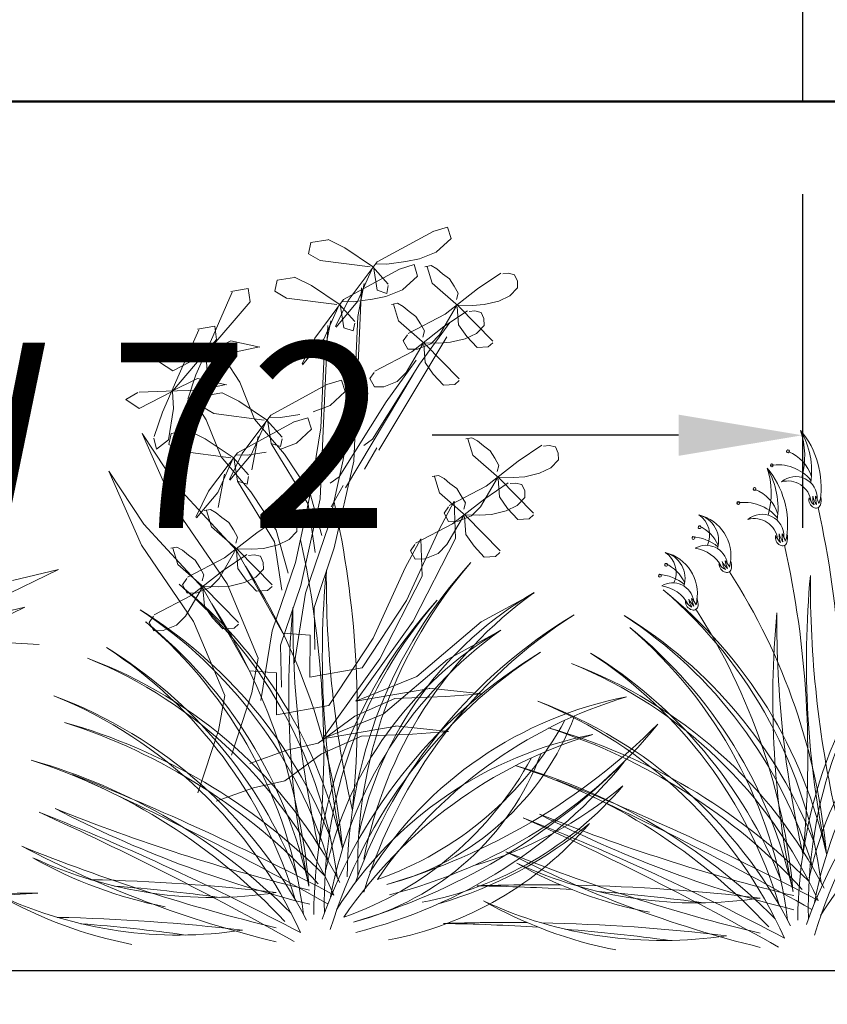
# Model space of a CAD drawing. Units: inches. Extents: x 89 to 490, y -59 to 378.
# Tile 11 of 20: x 374 to 400, y -24 to 7. Entities that reach past the tile are written whole.
import ezdxf

# ---------------------------------------------------------------- set-up
doc = ezdxf.new("R2010")
doc.units = ezdxf.units.IN
doc.header["$MEASUREMENT"] = 0
for name, color, linetype, lineweight in [('A-ANNO-DIMS', 2, 'Continuous', 18), ('L-PLNT', 94, 'Continuous', 18), ('L-PLNT-EDGE', 31, 'Continuous', 25), ('Outer Walls', 12, 'Continuous', 50), ('Windows', 171, 'Continuous', 25)]:
    doc.layers.add(name, color=color, linetype=linetype, lineweight=lineweight)
doc.layers.add('fl', color=73, linetype='Continuous', lineweight=9, true_color=0xa3d166)
doc.styles.get("Standard").update_dxf_attribs({"font": 'arial.ttf'})
doc.dimstyles.get("Standard").update_dxf_attribs({"dimtxt": 6, "dimasz": 4, "dimexe": 3, "dimexo": 3, "dimgap": 0.09, "dimtad": 0, "dimtih": 1, "dimtoh": 1, "dimdec": 1, "dimzin": 0, "dimdsep": 46, "dimlunit": 3, "dimtxsty": 'Standard', "dimcen": 0.09, "dimadec": 0, "dimazin": 0, "dimtfac": 1, "dimtdec": 1, "dimtofl": 0, "dimtmove": 0, "dimatfit": 3, "dimfxl": 1, "dimtolj": 1, "dimtzin": 0, "dimarcsym": 0})

# ---------------------------------------------------------------- blocks, each defined once
blk = doc.blocks.new('Window')
blk.add_lwpolyline([(588.369, 99.053), (588.369, 90.053), (516.369, 90.053), (516.369, 99.053)], close=True)
blk = doc.blocks.new('Plantation')
at = {"layer": 'fl'}
for p, q in [((609.786, 34.419), (611.6, 35.405)), ((612.07, 35.547), (611.594, 35.406)), ((612.182, 35.177), (612.07, 35.547)), ((608.2, 35.134), (607.643, 35.044)), ((608.206, 35.143), (608.75, 34.87)), ((611.699, 34.73), (612.182, 35.177)), ((607.643, 35.044), (607.57, 34.684)), ((608.75, 34.87), (609.645, 34.268)), ((611.158, 34.521), (611.699, 34.73)), ((607.57, 34.684), (607.946, 34.465)), ((607.946, 34.465), (609.569, 34.254)), ((608.856, 33.172), (609.786, 34.419)), ((610.099, 34.343), (610.721, 34.434)), ((610.721, 34.434), (611.158, 34.521)), ((608.702, 33.201), (610.516, 34.186)), ((609.151, 33.131), (609.649, 34.242)), ((609.645, 34.268), (610.151, 33.702)), ((609.795, 33.501), (609.675, 34.269)), ((609.754, 34.35), (610.099, 34.343)), ((610.986, 34.329), (610.51, 34.188)), ((611.099, 33.959), (610.986, 34.329)), ((611.337, 34.257), (611.537, 34.297)), ((611.405, 34.263), (611.569, 33.734)), ((611.537, 34.297), (611.721, 34.191)), ((611.721, 34.191), (611.905, 34.03)), ((606.56, 33.826), (606.486, 33.466)), ((607.116, 33.916), (606.56, 33.826)), ((607.122, 33.925), (607.666, 33.652)), ((610.615, 33.512), (611.099, 33.959)), ((611.905, 34.03), (612.126, 33.87)), ((612.126, 33.87), (612.276, 33.636)), ((613.034, 33.541), (613.794, 34.053)), ((614.034, 34.049), (613.852, 34.028)), ((614.235, 33.998), (614.034, 34.049)), ((614.329, 33.799), (614.235, 33.998)), ((614.333, 33.581), (614.329, 33.799)), ((605.062, 33.457), (605.625, 33.555)), ((605.625, 33.555), (605.683, 33.128)), ((606.486, 33.466), (606.862, 33.247)), ((607.666, 33.652), (608.561, 33.05)), ((609.28, 33.582), (609.036, 27.974)), ((609.166, 32.648), (609.372, 33.724)), ((610.102, 33.4), (609.795, 33.501)), ((610.074, 33.303), (610.615, 33.512)), ((610.151, 33.653), (610.102, 33.4)), ((611.569, 33.734), (612.421, 32.985)), ((611.992, 32.728), (613.034, 33.541)), ((612.276, 33.636), (612.408, 33.402)), ((614.083, 33.322), (614.333, 33.581)), ((604.472, 32.002), (605.104, 33.433)), ((606.862, 33.247), (608.486, 33.036)), ((607.772, 31.954), (608.702, 33.201)), ((608.447, 32.332), (608.856, 33.172)), ((609.015, 33.125), (609.638, 33.216)), ((609.638, 33.216), (610.074, 33.303)), ((612.408, 33.402), (612.356, 33.201)), ((613.251, 33.034), (613.722, 33.152)), ((613.722, 33.152), (614.083, 33.322)), ((605.683, 33.128), (604.255, 31.456)), ((608.067, 31.913), (608.565, 33.024)), ((608.461, 32.308), (609.151, 33.131)), ((608.561, 33.05), (609.067, 32.484)), ((608.711, 32.283), (608.591, 33.051)), ((608.67, 33.132), (609.015, 33.125)), ((610.254, 33.039), (610.453, 33.079)), ((610.321, 33.045), (610.485, 32.516)), ((610.453, 33.079), (610.637, 32.973)), ((610.637, 32.973), (610.821, 32.812)), ((611.812, 32.062), (612.36, 33)), ((611.95, 32.323), (612.71, 32.835)), ((612.379, 32.964), (612.425, 32.382)), ((612.414, 33.019), (612.869, 33.009)), ((612.421, 32.985), (613.528, 31.857)), ((612.95, 32.831), (612.768, 32.81)), ((612.869, 33.009), (613.251, 33.034)), ((613.151, 32.78), (612.95, 32.831)), ((608.082, 31.43), (608.288, 32.506)), ((609.053, 30.262), (609.166, 32.648)), ((610.485, 32.516), (611.337, 31.767)), ((610.798, 32.104), (611.992, 32.728)), ((610.821, 32.812), (611.043, 32.652)), ((611.043, 32.652), (611.192, 32.418)), ((613.245, 32.581), (613.151, 32.78)), ((613.249, 32.363), (613.245, 32.581)), ((603.389, 30.784), (604.02, 32.215)), ((603.978, 32.239), (604.541, 32.337)), ((604.541, 32.337), (604.599, 31.91)), ((608.196, 32.364), (607.953, 26.756)), ((609.018, 32.182), (608.711, 32.283)), ((609.067, 32.435), (609.018, 32.182)), ((610.908, 31.51), (611.95, 32.323)), ((611.163, 31.112), (612.138, 32.457)), ((611.192, 32.418), (611.324, 32.184)), ((611.324, 32.184), (611.273, 31.982)), ((612.425, 32.382), (612.687, 32.004)), ((612.999, 32.104), (613.249, 32.363)), ((604.599, 31.91), (603.171, 30.238)), ((603.931, 30.768), (604.472, 32.002)), ((607.364, 31.114), (607.772, 31.954)), ((607.378, 31.09), (608.067, 31.913)), ((609.85, 28.33), (612.039, 31.99)), ((610.775, 32.062), (610.633, 31.859)), ((611.526, 31.766), (611.812, 32.062)), ((612.167, 31.816), (612.638, 31.933)), ((612.638, 31.933), (612.999, 32.104)), ((612.687, 32.004), (613.02, 31.646)), ((605.064, 31.86), (604.217, 31.443)), ((605.998, 31.662), (605.064, 31.86)), ((605.122, 31.489), (605.991, 31.665)), ((610.633, 31.859), (610.784, 31.589)), ((610.728, 30.844), (611.276, 31.782)), ((610.784, 31.589), (611.093, 31.594)), ((611.093, 31.594), (611.526, 31.766)), ((611.295, 31.746), (611.341, 31.164)), ((611.33, 31.801), (611.785, 31.791)), ((611.337, 31.767), (612.445, 30.639)), ((611.785, 31.791), (612.167, 31.816)), ((613.02, 31.646), (613.384, 31.671)), ((613.384, 31.671), (613.527, 31.801)), ((603.137, 31.411), (602.752, 31.178)), ((603.18, 31.423), (604.054, 31.453)), ((603.184, 30.896), (604.242, 31.443)), ((604.054, 31.453), (605.122, 31.489)), ((604.29, 30.89), (604.255, 31.443)), ((604.887, 31.238), (605.349, 30.525)), ((607.969, 29.044), (608.082, 31.43)), ((609.714, 30.886), (610.908, 31.51)), ((610.079, 29.894), (611.054, 31.239)), ((602.752, 31.178), (603.184, 30.896)), ((609.641, 28.678), (611.163, 31.112)), ((611.341, 31.164), (611.603, 30.786)), ((602.847, 29.55), (603.389, 30.784)), ((603.98, 30.642), (603.133, 30.224)), ((603.666, 29.981), (603.931, 30.768)), ((604.914, 30.444), (603.98, 30.642)), ((604.131, 29.882), (604.29, 30.89)), ((608.638, 30.589), (608.162, 30.448)), ((608.751, 30.219), (608.638, 30.589)), ((608.766, 27.112), (610.956, 30.772)), ((609.692, 30.844), (609.55, 30.641)), ((609.55, 30.641), (609.7, 30.371)), ((610.443, 30.548), (610.728, 30.844)), ((611.603, 30.786), (611.936, 30.428)), ((602.97, 30.235), (604.038, 30.271)), ((604.038, 30.271), (604.907, 30.447)), ((605.349, 30.525), (605.828, 29.326)), ((606.354, 29.461), (608.168, 30.447)), ((609.7, 30.371), (610.009, 30.376)), ((610.009, 30.376), (610.443, 30.548)), ((611.936, 30.428), (612.3, 30.453)), ((612.3, 30.453), (612.443, 30.583)), ((602.053, 30.193), (601.668, 29.96)), ((601.668, 29.96), (602.1, 29.678)), ((602.096, 30.205), (602.97, 30.235)), ((602.1, 29.678), (603.158, 30.225)), ((603.206, 29.672), (603.171, 30.225)), ((603.804, 30.02), (604.265, 29.307)), ((604.212, 30.086), (604.138, 29.726)), ((604.768, 30.176), (604.212, 30.086)), ((604.774, 30.185), (605.318, 29.912)), ((608.267, 29.772), (608.751, 30.219)), ((608.692, 28.013), (609.053, 30.262)), ((603.047, 28.664), (603.206, 29.672)), ((603.653, 29.936), (603.735, 29.573)), ((603.735, 29.573), (604.131, 29.882)), ((604.138, 29.726), (604.514, 29.507)), ((605.318, 29.912), (606.213, 29.31)), ((607.726, 29.563), (608.267, 29.772)), ((608.558, 27.46), (610.079, 29.894)), ((602.582, 28.763), (602.847, 29.55)), ((604.514, 29.507), (606.138, 29.296)), ((605.424, 28.214), (606.354, 29.461)), ((605.828, 29.326), (606.79, 28.192)), ((606.322, 29.392), (606.667, 29.385)), ((606.667, 29.385), (607.29, 29.476)), ((607.554, 29.371), (607.079, 29.23)), ((607.667, 29.001), (607.554, 29.371)), ((604.265, 29.307), (604.744, 28.108)), ((605.27, 28.243), (607.084, 29.229)), ((605.719, 28.173), (606.217, 29.284)), ((606.213, 29.31), (606.719, 28.744)), ((606.363, 28.543), (606.244, 29.311)), ((607.183, 28.554), (607.667, 29.001)), ((607.608, 26.795), (607.969, 29.044)), ((603.251, 26.467), (602.197, 28.861)), ((602.197, 28.861), (603.325, 27.15)), ((602.569, 28.718), (602.651, 28.355)), ((603.128, 28.868), (603.054, 28.508)), ((603.684, 28.958), (603.128, 28.868)), ((603.69, 28.967), (604.234, 28.694)), ((604.234, 28.694), (605.13, 28.092)), ((605.734, 27.69), (605.94, 28.766)), ((606.719, 28.695), (606.67, 28.442)), ((609.357, 28.474), (609.641, 28.678)), ((612.657, 28.689), (612.857, 28.729)), ((612.724, 28.695), (612.888, 28.166)), ((612.857, 28.729), (613.04, 28.623)), ((602.651, 28.355), (603.047, 28.664)), ((603.054, 28.508), (603.43, 28.289)), ((606.363, 28.543), (607.558, 26.582)), ((606.67, 28.442), (606.363, 28.543)), ((606.643, 28.345), (607.183, 28.554)), ((609.383, 27.707), (609.78, 28.397)), ((613.04, 28.623), (613.225, 28.462)), ((613.225, 28.462), (613.446, 28.302)), ((614.353, 27.973), (615.114, 28.485)), ((615.353, 28.481), (615.172, 28.46)), ((615.554, 28.43), (615.353, 28.481)), ((615.649, 28.231), (615.554, 28.43)), ((603.43, 28.289), (605.054, 28.078)), ((604.341, 26.996), (605.27, 28.243)), ((604.635, 26.955), (605.134, 28.066)), ((604.744, 28.108), (605.706, 26.974)), ((605.016, 27.374), (605.424, 28.214)), ((605.03, 27.35), (605.719, 28.173)), ((605.13, 28.092), (605.635, 27.526)), ((605.279, 27.325), (605.16, 28.093)), ((605.238, 28.174), (605.583, 28.167)), ((605.583, 28.167), (606.206, 28.258)), ((606.79, 28.192), (607.61, 26.956)), ((612.888, 28.166), (613.74, 27.418)), ((613.446, 28.302), (613.596, 28.068)), ((613.596, 28.068), (613.727, 27.834)), ((615.653, 28.013), (615.649, 28.231)), ((608.229, 25.907), (608.692, 28.013)), ((609.036, 27.974), (608.403, 25.161)), ((613.312, 27.16), (614.353, 27.973)), ((613.727, 27.834), (613.676, 27.633)), ((615.042, 27.584), (615.402, 27.754)), ((615.402, 27.754), (615.653, 28.013)), ((602.168, 25.249), (601.114, 27.643)), ((601.114, 27.643), (602.241, 25.932)), ((604.65, 26.472), (604.857, 27.548)), ((605.635, 27.477), (605.587, 27.224)), ((608.273, 27.256), (608.558, 27.46)), ((611.573, 27.471), (611.773, 27.511)), ((611.641, 27.477), (611.804, 26.948)), ((611.773, 27.511), (611.957, 27.405)), ((611.957, 27.405), (612.141, 27.244)), ((613.132, 26.494), (613.68, 27.432)), ((613.734, 27.451), (614.189, 27.441)), ((613.74, 27.418), (614.848, 26.289)), ((614.189, 27.441), (614.571, 27.466)), ((614.571, 27.466), (615.042, 27.584)), ((603.325, 27.15), (605.243, 25.076)), ((605.279, 27.325), (606.475, 25.364)), ((605.587, 27.224), (605.279, 27.325)), ((608.299, 26.489), (608.696, 27.179)), ((612.118, 26.536), (613.312, 27.16)), ((612.141, 27.244), (612.362, 27.084)), ((612.362, 27.084), (612.512, 26.85)), ((613.269, 26.755), (614.03, 27.267)), ((613.699, 27.396), (613.745, 26.814)), ((614.269, 27.263), (614.088, 27.242)), ((614.47, 27.212), (614.269, 27.263)), ((614.565, 27.013), (614.47, 27.212)), ((603.932, 26.156), (604.341, 26.996)), ((603.946, 26.132), (604.635, 26.955)), ((605.706, 26.974), (606.526, 25.738)), ((607.145, 24.689), (607.608, 26.795)), ((607.61, 26.956), (607.998, 25.559)), ((611.804, 26.948), (612.656, 26.2)), ((612.512, 26.85), (612.643, 26.616)), ((613.745, 26.814), (614.006, 26.437)), ((614.319, 26.536), (614.569, 26.795)), ((614.569, 26.795), (614.565, 27.013)), ((604.94, 23.997), (603.251, 26.467)), ((607.953, 26.756), (607.319, 23.943)), ((607.558, 26.582), (607.791, 25.014)), ((611.783, 25.737), (612.286, 26.678)), ((612.095, 26.494), (611.953, 26.291)), ((612.228, 25.942), (613.269, 26.755)), ((612.286, 26.678), (612.328, 25.464)), ((612.643, 26.616), (612.592, 26.415)), ((612.846, 26.198), (613.132, 26.494)), ((613.958, 26.366), (614.319, 26.536)), ((604.202, 26.369), (604.401, 26.409)), ((604.269, 26.376), (604.433, 25.846)), ((604.401, 26.409), (604.585, 26.303)), ((604.585, 26.303), (604.77, 26.142)), ((604.77, 26.142), (604.991, 25.982)), ((605.898, 25.653), (606.658, 26.165)), ((606.898, 26.161), (606.717, 26.14)), ((607.099, 26.11), (606.898, 26.161)), ((611.953, 26.291), (612.103, 26.021)), ((612.048, 25.276), (612.596, 26.214)), ((612.413, 26.026), (612.846, 26.198)), ((612.615, 26.178), (612.661, 25.596)), ((612.65, 26.233), (613.105, 26.223)), ((612.656, 26.2), (613.764, 25.071)), ((613.105, 26.223), (613.487, 26.248)), ((613.487, 26.248), (613.958, 26.366)), ((614.006, 26.437), (614.34, 26.078)), ((614.704, 26.103), (614.847, 26.233)), ((602.241, 25.932), (604.159, 23.858)), ((604.433, 25.846), (605.285, 25.098)), ((604.991, 25.982), (605.141, 25.748)), ((607.194, 25.912), (607.099, 26.11)), ((607.197, 25.693), (607.194, 25.912)), ((607.478, 23.694), (608.229, 25.907)), ((611.034, 25.318), (612.228, 25.942)), ((612.103, 26.021), (612.413, 26.026)), ((614.34, 26.078), (614.704, 26.103)), ((604.856, 24.84), (605.898, 25.653)), ((605.141, 25.748), (605.272, 25.514)), ((605.272, 25.514), (605.221, 25.313)), ((606.526, 25.738), (606.914, 24.341)), ((606.947, 25.434), (607.197, 25.693)), ((610.743, 23.465), (611.783, 25.737)), ((612.661, 25.596), (612.923, 25.219)), ((603.856, 22.778), (602.168, 25.249)), ((603.118, 25.151), (603.318, 25.191)), ((603.318, 25.191), (603.501, 25.085)), ((606.115, 25.146), (606.586, 25.264)), ((606.475, 25.364), (606.707, 23.796)), ((606.586, 25.264), (606.947, 25.434)), ((610.7, 24.519), (611.202, 25.46)), ((611.011, 25.276), (610.869, 25.073)), ((612.328, 25.464), (610.96, 22.792)), ((611.202, 25.46), (611.244, 24.246)), ((611.762, 24.98), (612.048, 25.276)), ((612.923, 25.219), (613.256, 24.86)), ((603.185, 25.158), (603.349, 24.628)), ((603.501, 25.085), (603.686, 24.924)), ((603.686, 24.924), (603.907, 24.764)), ((604.677, 24.174), (605.224, 25.112)), ((604.814, 24.435), (605.575, 24.947)), ((605.243, 25.076), (606.744, 22.405)), ((605.243, 25.076), (605.29, 24.494)), ((605.279, 25.132), (605.734, 25.121)), ((605.285, 25.098), (606.393, 23.969)), ((605.814, 24.943), (605.633, 24.922)), ((605.734, 25.121), (606.115, 25.146)), ((606.015, 24.892), (605.814, 24.943)), ((606.11, 24.694), (606.015, 24.892)), ((608.403, 25.161), (607.753, 23.236)), ((610.869, 25.073), (611.02, 24.803)), ((611.329, 24.808), (611.762, 24.98)), ((613.256, 24.86), (613.62, 24.885)), ((613.62, 24.885), (613.763, 25.015)), ((603.349, 24.628), (604.201, 23.88)), ((603.662, 24.216), (604.856, 24.84)), ((603.907, 24.764), (604.057, 24.53)), ((606.113, 24.475), (606.11, 24.694)), ((606.394, 22.476), (607.145, 24.689)), ((611.02, 24.803), (611.329, 24.808)), ((599.485, 24.463), (597.342, 23.428)), ((597.995, 24.105), (599.485, 24.463)), ((603.772, 23.622), (604.814, 24.435)), ((604.057, 24.53), (604.188, 24.296)), ((604.188, 24.296), (604.137, 24.095)), ((605.29, 24.494), (605.551, 24.117)), ((605.502, 24.046), (605.863, 24.216)), ((605.863, 24.216), (606.113, 24.475)), ((609.659, 22.247), (610.7, 24.519)), ((611.244, 24.246), (609.876, 21.574)), ((603.64, 24.174), (603.498, 23.972)), ((603.498, 23.972), (603.648, 23.701)), ((604.195, 23.914), (604.65, 23.903)), ((604.391, 23.878), (604.677, 24.174)), ((604.65, 23.903), (605.031, 23.928)), ((605.945, 21.6), (604.94, 23.997)), ((605.031, 23.928), (605.502, 24.046)), ((605.551, 24.117), (605.885, 23.758)), ((606.248, 23.783), (606.392, 23.913)), ((607.319, 23.943), (606.669, 22.018)), ((602.578, 22.998), (603.772, 23.622)), ((603.593, 22.956), (604.141, 23.894)), ((603.648, 23.701), (603.957, 23.706)), ((603.957, 23.706), (604.391, 23.878)), ((604.159, 23.858), (605.66, 21.187)), ((604.159, 23.858), (604.206, 23.276)), ((604.201, 23.88), (605.309, 22.751)), ((605.885, 23.758), (606.248, 23.783)), ((607.117, 21.446), (607.478, 23.694)), ((613.149, 22.769), (614.867, 23.703)), ((604.206, 23.276), (604.467, 22.899)), ((609.31, 21.277), (610.743, 23.465)), ((598.401, 23.245), (596.258, 22.21)), ((596.911, 22.887), (598.401, 23.245)), ((602.556, 22.956), (602.414, 22.754)), ((603.307, 22.66), (603.593, 22.956)), ((607.753, 23.236), (607.777, 21.87)), ((602.414, 22.754), (602.564, 22.483)), ((602.874, 22.488), (603.307, 22.66)), ((604.861, 20.382), (603.856, 22.778)), ((604.467, 22.899), (604.801, 22.54)), ((605.164, 22.565), (605.308, 22.695)), ((610.96, 22.792), (609.104, 20.201)), ((611.07, 20.997), (613.149, 22.769)), ((602.564, 22.483), (602.874, 22.488)), ((604.801, 22.54), (605.164, 22.565)), ((606.033, 20.228), (606.394, 22.476)), ((606.744, 22.405), (607.621, 22.338)), ((607.621, 22.338), (607.619, 20.977)), ((612.065, 21.551), (613.783, 22.485)), ((595.368, 22.229), (598.862, 22.04)), ((606.669, 22.018), (606.693, 20.652)), ((608.227, 20.059), (609.659, 22.247)), ((605.74, 20.475), (605.945, 21.6)), ((609.876, 21.574), (608.02, 18.983)), ((609.986, 19.779), (612.065, 21.551)), ((605.66, 21.187), (606.538, 21.12)), ((606.538, 21.12), (606.535, 19.759)), ((607.619, 20.977), (609.31, 21.277)), ((609.104, 20.201), (611.07, 20.997)), ((605.08, 18.459), (605.74, 20.475)), ((611.493, 20.611), (609.106, 20.206)), ((611.472, 20.622), (613.18, 20.437)), ((613.18, 20.437), (612.016, 20.349)), ((604.657, 19.257), (604.861, 20.382)), ((610.365, 20.293), (609.072, 19.714)), ((612.016, 20.349), (610.365, 20.293)), ((606.535, 19.759), (608.227, 20.059)), ((608.02, 18.983), (609.986, 19.779)), ((609.072, 19.714), (607.886, 18.847)), ((603.996, 17.241), (604.657, 19.257)), ((610.409, 19.393), (608.022, 18.988)), ((610.932, 19.131), (609.281, 19.074)), ((610.388, 19.404), (612.096, 19.219)), ((612.096, 19.219), (610.932, 19.131)), ((607.886, 18.847), (606.873, 18.618)), ((609.281, 19.074), (607.988, 18.496)), ((606.873, 18.618), (605.673, 18.188)), ((607.988, 18.496), (606.803, 17.629)), ((606.803, 17.629), (605.789, 17.4)), ((605.789, 17.4), (604.589, 16.97))]:
    blk.add_line(p, q, dxfattribs=at)
for centre, radius, start, end in [((621.293, 27.138), 2.854, 351.4134, 39.8275), ((621.008, 28.148), 2.608, 344.3064, 18.279), ((621.238, 27.658), 2.6, 351.5096, 30.1949), ((623.078, 28.288), 0.0459, 7.5892, 187.5892), ((623.078, 28.288), 0.0459, 187.5892, 7.5892), ((622.642, 27.116), 1.243, 16.8512, 68.8014), ((620.209, 25.92), 2.854, 351.4134, 39.8275), ((619.925, 26.93), 2.608, 344.3064, 18.279), ((620.154, 26.44), 2.6, 351.5096, 30.1949), ((622.552, 27.835), 0.0459, 7.5892, 187.5892), ((622.75, 26.467), 1.386, 39.5069, 100.1323), ((622.552, 27.835), 0.0459, 187.5892, 7.5892), ((623.323, 26.769), 0.701, 357.4175, 130.8703), ((621.994, 27.07), 0.0459, 7.5892, 187.5892), ((623.073, 26.575), 0.754, 6.9832, 106.1055), ((621.994, 27.07), 0.0459, 187.5892, 7.5892), ((621.558, 25.898), 1.243, 16.8512, 68.8014), ((624.041, 26.724), 0.289, 168.1654, 242.3938), ((624.313, 27.002), 0.596, 201.5294, 228.9216), ((624.439, 26.778), 0.565, 174.5103, 203.5444), ((624.591, 26.998), 0.733, 193.0983, 215.538), ((625.276, 26.832), 1.308, 179.8013, 191.4565), ((623.391, 26.451), 0.694, 12.1333, 33.7421), ((623.12, 27.043), 1.049, 334.86, 346.6738), ((623.552, 26.716), 0.595, 343.9406, 8.2206), ((577.655, 19.804), 31.492, 354.2791, 12.5427), ((621.468, 26.617), 0.0459, 7.5892, 187.5892), ((621.666, 25.249), 1.386, 39.5069, 100.1323), ((621.468, 26.617), 0.0459, 187.5892, 7.5892), ((623.98, 26.6), 0.151, 241.146, 341.1111), ((593.308, 19.626), 31.492, 354.2791, 12.5427), ((619.968, 25.398), 0.863, 342.816, 75.0201), ((619.75, 25.572), 0.793, 335.7976, 56.2278), ((619.863, 24.903), 1.368, 349.633, 76.1366), ((622.239, 25.551), 0.701, 357.4175, 130.8703), ((620.219, 25.831), 0.0459, 19.649, 199.649), ((620.219, 25.831), 0.0459, 199.649, 19.649), ((619.684, 24.745), 1.243, 24.0842, 65.3008), ((621.989, 25.357), 0.754, 6.9832, 106.1055), ((620.019, 25.484), 0.0459, 19.649, 199.649), ((620.019, 25.484), 0.0459, 199.649, 19.649), ((619.924, 24.133), 1.386, 50.416, 87.3549), ((622.957, 25.506), 0.289, 168.1654, 242.3938), ((623.229, 25.784), 0.596, 201.5294, 228.9216), ((623.355, 25.56), 0.565, 174.5103, 203.5444), ((623.507, 25.78), 0.733, 193.0983, 215.538), ((624.192, 25.614), 1.308, 179.8013, 191.4565), ((622.307, 25.233), 0.694, 12.1333, 33.7421), ((622.036, 25.825), 1.049, 334.86, 346.6738), ((622.468, 25.498), 0.595, 343.9406, 8.2206), ((576.571, 18.586), 31.492, 354.2791, 12.5427), ((620.426, 24.552), 0.696, 9.2042, 120.225), ((622.896, 25.382), 0.151, 241.146, 341.1111), ((592.224, 18.408), 31.492, 354.2791, 12.5427), ((618.884, 24.18), 0.863, 342.816, 75.0201), ((618.666, 24.354), 0.793, 335.7976, 56.2278), ((618.779, 23.685), 1.368, 349.633, 76.1366), ((619.911, 24.011), 1.154, 27.9293, 81.8071), ((588.534, 13.624), 20.216, 5.151, 32.7872), ((624.023, 14.414), 15.201, 137.4916, 179.6099), ((624.085, 14.904), 14.921, 139.0392, 181.297), ((619.135, 24.613), 0.0459, 19.649, 199.649), ((619.135, 24.613), 0.0459, 199.649, 19.649), ((618.6, 23.527), 1.243, 24.0842, 65.3008), ((621.134, 24.654), 0.289, 180.2252, 254.4537), ((621.341, 24.982), 0.596, 213.5892, 240.9815), ((621.512, 24.79), 0.565, 186.5701, 215.6042), ((621.614, 25.037), 0.733, 205.1582, 227.5978), ((620.555, 24.251), 0.694, 24.1932, 45.802), ((622.319, 25.017), 1.308, 191.8611, 203.5164), ((620.166, 24.773), 1.049, 346.9198, 358.7337), ((620.657, 24.543), 0.595, 356.0005, 20.2804), ((637.911, 21.649), 29.894, 174.6174, 191.9895), ((642.136, 24.184), 33.989, 179.5471, 192.7817), ((618.936, 24.266), 0.0459, 19.649, 199.649), ((618.936, 24.266), 0.0459, 199.649, 19.649), ((618.841, 22.915), 1.386, 50.416, 87.3549), ((621.1, 24.52), 0.151, 253.2058, 353.1709), ((604.187, 13.446), 20.216, 5.151, 32.7872), ((653.564, 21.471), 29.894, 174.6174, 191.9895), ((657.789, 24.006), 33.989, 179.5471, 192.7817), ((593.69, 12.647), 14.921, 7.1968, 49.4547), ((593.823, 12.171), 15.201, 12.4122, 51.0023), ((619.342, 23.334), 0.696, 9.2042, 120.225), ((618.827, 22.793), 1.154, 27.9293, 81.8071), ((620.943, 13.352), 12.017, 120.3536, 167.8423), ((622.972, 12.48), 13.856, 125.7805, 169.1581), ((609.343, 12.469), 14.921, 7.1968, 49.4547), ((609.476, 11.993), 15.201, 12.4122, 51.0023), ((587.45, 12.406), 20.216, 5.151, 32.7872), ((622.939, 13.196), 15.201, 137.4916, 179.6099), ((623.001, 13.686), 14.921, 139.0392, 181.297), ((620.05, 23.436), 0.289, 180.2252, 254.4537), ((620.257, 23.764), 0.596, 213.5892, 240.9815), ((620.428, 23.572), 0.565, 186.5701, 215.6042), ((620.53, 23.819), 0.733, 205.1582, 227.5978), ((619.471, 23.033), 0.694, 24.1932, 45.802), ((621.235, 23.799), 1.308, 191.8611, 203.5164), ((620.016, 23.302), 0.151, 253.2058, 353.1709), ((619.082, 23.555), 1.049, 346.9198, 358.7337), ((619.573, 23.325), 0.595, 356.0005, 20.2804), ((638.593, 13.018), 15.201, 137.4916, 179.6099), ((638.654, 13.508), 14.921, 139.0392, 181.297), ((593.941, 10.681), 14.921, 16.8321, 56.7339), ((594.134, 10.226), 15.201, 21.5651, 58.2814), ((636.827, 20.431), 29.894, 174.6174, 191.9895), ((641.052, 22.966), 33.989, 179.5471, 192.7817), ((624.767, 8.759), 16.642, 121.1471, 160.292), ((624.9, 9.316), 16.239, 122.567, 163.1344), ((609.594, 10.503), 14.921, 16.8321, 56.7339), ((609.787, 10.048), 15.201, 21.5651, 58.2814), ((603.103, 12.228), 20.216, 5.151, 32.7872), ((652.48, 20.253), 29.894, 174.6174, 191.9895), ((656.705, 22.788), 33.989, 179.5471, 192.7817), ((592.606, 11.429), 14.921, 7.1968, 49.4547), ((592.739, 10.953), 15.201, 12.4122, 51.0023), ((619.859, 12.134), 12.017, 120.3536, 167.8423), ((621.888, 11.262), 13.856, 125.7805, 169.1581), ((608.259, 11.251), 14.921, 7.1968, 49.4547), ((608.392, 10.775), 15.201, 12.4122, 51.0023), ((635.513, 11.956), 12.017, 120.3536, 167.8423), ((637.541, 11.084), 13.856, 125.7805, 169.1581), ((592.857, 9.463), 14.921, 16.8321, 56.7339), ((593.05, 9.008), 15.201, 21.5651, 58.2814), ((623.683, 7.541), 16.642, 121.1471, 160.292), ((623.816, 8.098), 16.239, 122.567, 163.1344), ((608.51, 9.285), 14.921, 16.8321, 56.7339), ((608.703, 8.83), 15.201, 21.5651, 58.2814), ((595.079, 7.366), 15.201, 27.2807, 69.4256), ((594.802, 7.775), 14.921, 24.3637, 67.878), ((610.732, 7.188), 15.201, 27.2807, 69.4256), ((610.455, 7.597), 14.921, 24.3637, 67.878), ((639.336, 7.363), 16.642, 121.1471, 160.292), ((639.469, 7.92), 16.239, 122.567, 163.1344), ((593.995, 6.148), 15.201, 27.2807, 69.4256), ((593.718, 6.557), 14.921, 24.3637, 67.878), ((620.256, 7.932), 12.64, 100.96, 147.8088), ((622.139, 6.06), 14.911, 106.7083, 145.8338), ((609.648, 5.97), 15.201, 27.2807, 69.4256), ((609.371, 6.379), 14.921, 24.3637, 67.878), ((594.461, 1.044), 19.194, 44.7494, 74.2143), ((593.838, 1.281), 19.147, 42.8064, 72.2288), ((606.162, 24.859), 11.042, 289.2472, 331.4766), ((607.868, 22.866), 8.88, 284.6053, 339.2893), ((604.392, 33.925), 20.466, 286.2137, 315.0057), ((606.218, 29.775), 16.324, 284.0723, 320.7861), ((619.172, 6.714), 12.64, 100.96, 147.8088), ((621.055, 4.842), 14.911, 106.7083, 145.8338), ((610.114, 0.866), 19.194, 44.7494, 74.2143), ((609.491, 1.103), 19.147, 42.8064, 72.2288), ((634.825, 6.536), 12.64, 100.96, 147.8088), ((606.784, 21.648), 8.88, 284.6053, 339.2893), ((593.377, -0.174), 19.194, 44.7494, 74.2143), ((592.754, 0.063), 19.147, 42.8064, 72.2288), ((605.078, 23.641), 11.042, 289.2472, 331.4766), ((603.308, 32.707), 20.466, 286.2137, 315.0057), ((605.134, 28.557), 16.324, 284.0723, 320.7861), ((609.03, -0.352), 19.194, 44.7494, 74.2143), ((608.408, -0.115), 19.147, 42.8064, 72.2288), ((555.414, -80.232), 107.696, 60.65352, 65.57668), ((569.549, -59.2), 82.807, 62.02355, 68.46556), ((571.067, -80.41), 107.696, 60.65352, 65.57668), ((585.202, -59.378), 82.807, 62.02355, 68.46556), ((609.131, 24.823), 11.325, 280.7497, 319.4803), ((609.267, 27.505), 13.137, 285.9859, 310.1616), ((554.33, -81.45), 107.696, 60.65352, 65.57668), ((568.465, -60.418), 82.807, 62.02355, 68.46556), ((616.347, 49.35), 36.77, 242.5259, 256.2554), ((621.334, 70.997), 58.541, 247.9781, 256.44), ((569.983, -81.628), 107.696, 60.65352, 65.57668), ((584.118, -60.596), 82.807, 62.02355, 68.46556), ((632, 49.172), 36.77, 242.5259, 256.2554), ((636.987, 70.819), 58.541, 247.9781, 256.44), ((608.047, 23.605), 11.325, 280.7497, 319.4803), ((608.184, 26.287), 13.137, 285.9859, 310.1616), ((615.263, 48.132), 36.77, 242.5259, 256.2554), ((620.25, 69.779), 58.541, 247.9781, 256.44), ((630.916, 47.954), 36.77, 242.5259, 256.2554), ((635.903, 69.601), 58.541, 247.9781, 256.44), ((605.614, 27.338), 14.044, 240.3144, 259.0249), ((604.452, 27.557), 13.704, 244.9915, 278.6666), ((621.267, 27.16), 14.044, 240.3144, 259.0249), ((620.105, 27.379), 13.704, 244.9915, 278.6666), ((599.331, -45.918), 60.356, 83.15791, 88.86091), ((596.497, -45.986), 60.398, 82.20958, 85.44376), ((614.984, -46.096), 60.356, 89.2944, 91.86186), ((612.15, -46.164), 60.398, 86.26075, 89.17238), ((614.984, -46.096), 60.356, 83.15791, 88.86091), ((612.15, -46.164), 60.398, 82.20958, 85.44376), ((601.803, -46.334), 60.398, 92.82762, 95.73925), ((598.969, -46.365), 60.356, 90.13814, 92.7056), ((604.53, 26.12), 14.044, 240.3144, 259.0249), ((603.368, 26.339), 13.704, 244.9915, 278.6666), ((620.183, 25.942), 14.044, 240.3144, 259.0249), ((619.021, 26.161), 13.704, 244.9915, 278.6666), ((598.247, -47.136), 60.356, 83.15791, 88.86091), ((595.414, -47.204), 60.398, 82.20958, 85.44376), ((613.9, -47.314), 60.356, 89.2944, 91.86186), ((611.067, -47.382), 60.398, 86.26075, 89.17238), ((613.9, -47.314), 60.356, 83.15791, 88.86091), ((611.067, -47.382), 60.398, 82.20958, 85.44376)]:
    blk.add_arc(centre, radius, start, end, dxfattribs=at)
blk = doc.blocks.new('*D36')
at = {"layer": 'A-ANNO-DIMS', "color": 0, "lineweight": -2, "transparency": 16777216}
for p, q in [((327.654, 1.741), (327.654, -9.059)), ((399.654, 1.741), (399.654, -9.059)), ((331.654, -6.059), (339.621, -6.059)), ((395.654, -6.059), (387.687, -6.059))]:
    blk.add_line(p, q, dxfattribs=at)
at = {"layer": 'A-ANNO-DIMS', "color": 0, "transparency": 16777216}
for points in [[(331.654, -5.392), (331.654, -6.725), (327.654, -6.059)], [(395.654, -5.392), (395.654, -6.725), (399.654, -6.059)]]:
    blk.add_solid(points, dxfattribs=at)
at = {"layer": 'Defpoints', "color": 0, "transparency": 16777216}
for p in [(327.654, 4.741), (399.654, 4.741), (399.654, -6.059)]:
    blk.add_point(p, dxfattribs=at)
at = {"layer": 'A-ANNO-DIMS', "color": 0, "transparency": 16777216, "insert": (363.654, -6.059), "char_height": 6, "attachment_point": 5}
blk.add_mtext('\\A1;WINDOW 72', dxfattribs=at)
blk = doc.blocks.new('*D37')
at = {"layer": 'A-ANNO-DIMS', "color": 0, "lineweight": -2, "transparency": 16777216}
for p, q in [((410.454, 13.741), (410.454, 17.741)), ((410.454, 17.741), (414.454, 17.741)), ((402.654, 13.741), (413.454, 13.741)), ((410.454, 8.741), (410.454, 9.741)), ((402.654, 4.741), (413.454, 4.741))]:
    blk.add_line(p, q, dxfattribs=at)
at = {"layer": 'A-ANNO-DIMS', "color": 0, "transparency": 16777216}
for points in [[(409.787, 9.741), (411.121, 9.741), (410.454, 13.741)], [(409.787, 8.741), (411.121, 8.741), (410.454, 4.741)]]:
    blk.add_solid(points, dxfattribs=at)
at = {"layer": 'Defpoints', "color": 0, "transparency": 16777216}
for p in [(399.654, 13.741), (410.454, 13.741), (399.654, 4.741)]:
    blk.add_point(p, dxfattribs=at)
at = {"layer": 'A-ANNO-DIMS', "color": 0, "transparency": 16777216, "insert": (416.517, 17.741), "char_height": 6, "attachment_point": 5}
blk.add_mtext('\\A1;9', dxfattribs=at)
blk = doc.blocks.new('*D48')
at = {"layer": 'A-ANNO-DIMS', "color": 0, "lineweight": -2, "transparency": 16777216}
for p, q in [((127.441, 10.741), (127.441, -49.809)), ((459.441, -29.659), (459.441, -49.809)), ((131.441, -46.809), (286.756, -46.809)), ((455.441, -46.809), (300.127, -46.809))]:
    blk.add_line(p, q, dxfattribs=at)
at = {"layer": 'A-ANNO-DIMS', "color": 0, "transparency": 16777216}
for points in [[(131.441, -46.143), (131.441, -47.476), (127.441, -46.809)], [(455.441, -46.143), (455.441, -47.476), (459.441, -46.809)]]:
    blk.add_solid(points, dxfattribs=at)
at = {"layer": 'Defpoints', "color": 0, "transparency": 16777216}
for p in [(127.441, 13.741), (459.441, -26.659), (459.441, -46.809)]:
    blk.add_point(p, dxfattribs=at)
at = {"layer": 'A-ANNO-DIMS', "color": 0, "transparency": 16777216, "insert": (293.441, -46.809), "char_height": 6, "attachment_point": 5}
blk.add_mtext('\\A1;332', dxfattribs=at)

msp = doc.modelspace()

# ---------------------------------------------------------------- linework, layer by layer
at = {"layer": 'L-PLNT-EDGE'}
msp.add_line((459.4414, -23.3886), (265.4414, -23.3886), dxfattribs=at)
at = {"layer": 'Outer Walls'}
msp.add_lwpolyline([(214.6478, 67.7413), (265.4414, 67.7413), (265.4414, 4.7413), (459.4414, 4.7413), (459.4414, 353.7413), (127.4414, 353.7413), (127.4414, 13.7413)], dxfattribs=at)

# ---------------------------------------------------------------- block references
at = {"layer": 'L-PLNT'}
msp.add_blockref('Plantation', (-223.8856, -34.8668), dxfattribs=at)
at = {"layer": 'Windows'}
msp.add_blockref('Window', (-188.7147, -85.3119), dxfattribs=at)

# ---------------------------------------------------------------- dimensions: what is measured, and where the dimension line sits
at = {"layer": 'A-ANNO-DIMS'}
dim = msp.add_linear_dim(base=(410.4539, 13.7413), p1=(399.6539, 4.7413), p2=(399.6539, 13.7413), angle=90, dimstyle='Standard', override={"dimdec": 0, "dimlfac": 1, "dimrnd": 0, "dimzin": 0, "dimdsep": 46, "dimlunit": 2}, dxfattribs=at)
dim.commit()
dim.dimension.update_dxf_attribs({"geometry": '*D37', "text_midpoint": (416.5166, 17.7413)})
dim = msp.add_linear_dim(base=(459.4414, -46.8094), p1=(127.4414, 13.7413), p2=(459.4414, -26.6594), dimstyle='Standard', override={"dimdec": 0, "dimlfac": 1, "dimrnd": 0, "dimzin": 0, "dimdsep": 46, "dimlunit": 2}, dxfattribs=at)
dim.commit()
dim.dimension.update_dxf_attribs({"geometry": '*D48', "text_midpoint": (293.4414, -46.8094)})
dim = msp.add_linear_dim(base=(399.6539, -6.0587), p1=(327.6539, 4.7413), p2=(399.6539, 4.7413), text='WINDOW <>', dimstyle='Standard', override={"dimdec": 0, "dimlfac": 1, "dimrnd": 0, "dimzin": 0, "dimdsep": 46, "dimlunit": 2}, dxfattribs=at)
dim.commit()
dim.dimension.update_dxf_attribs({"geometry": '*D36', "text_midpoint": (363.6539, -6.0587)})

doc.saveas('drawing.dxf')
